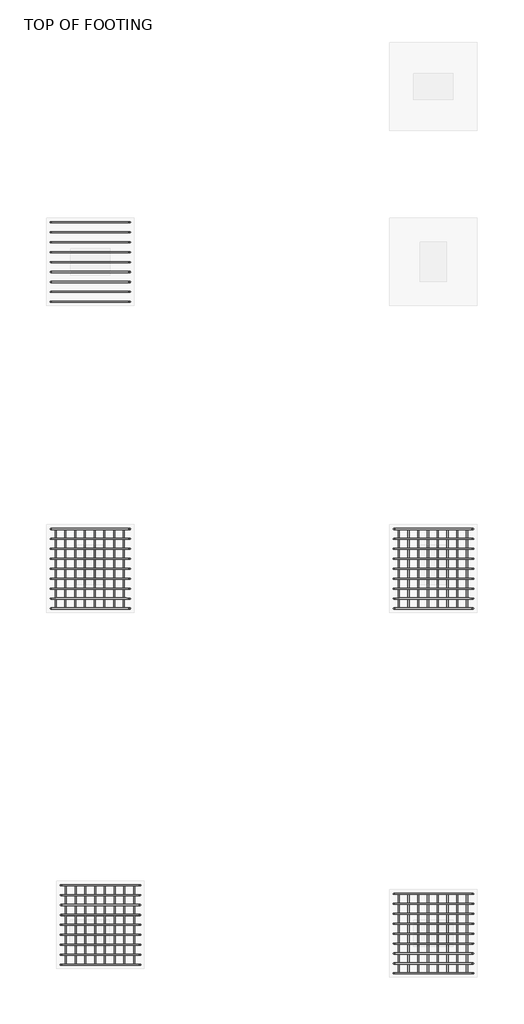
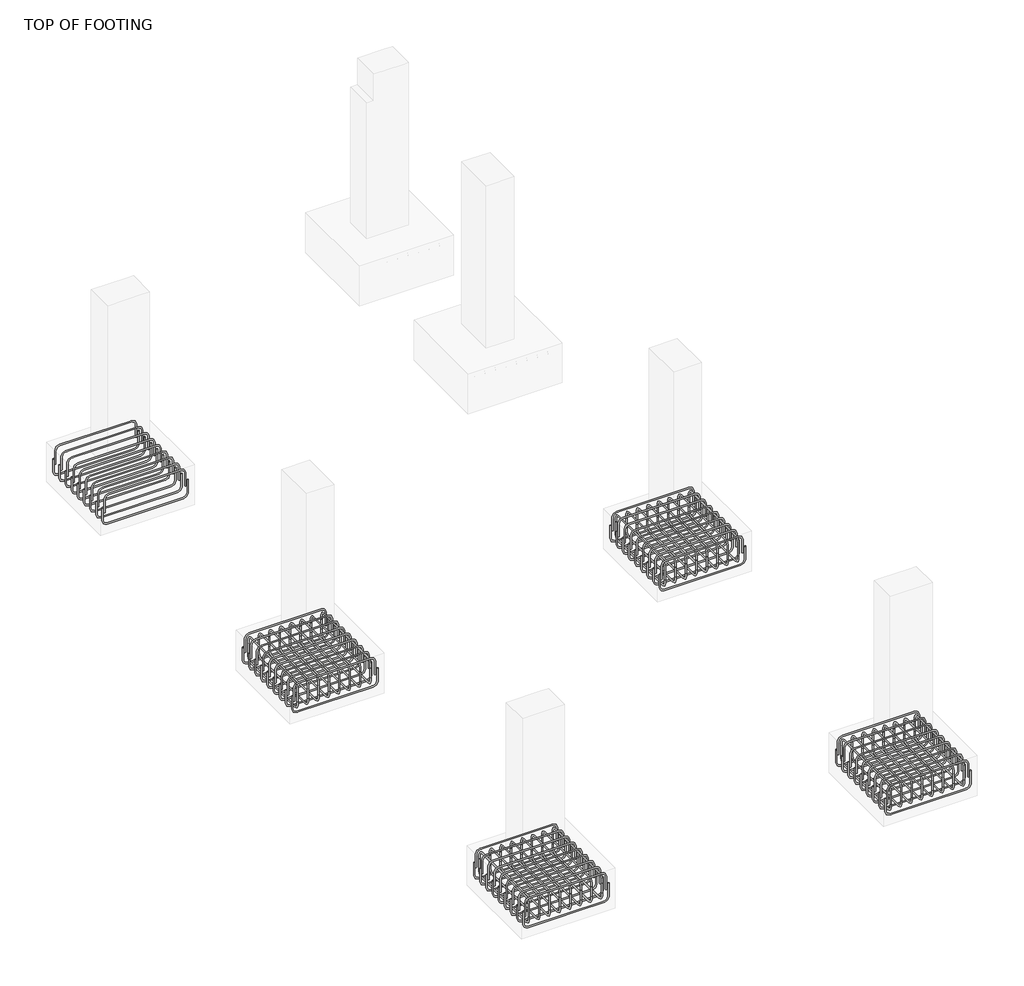
# One storey, part 3 of 20: 18 reinforcing bars.
"""IFC4 building model written with IfcOpenShell, lengths in millimetres."""

from ifc_helpers import new_model, si_unit, point, frame, origin, place, context, project, spatial, polyline, circle_curve, trimmed, segment, composite_curve, source, transform, mapped, element, save
from ifc_brep_helpers import swept_disk

model = new_model("IFC4")

# Units and contexts
model_context = context("Model", 3, world=origin())
ifc_project = project(units=[si_unit("LENGTHUNIT", "METRE", prefix="MILLI")], contexts=[model_context])

# Site, building, storey
site = spatial("IfcSite", under=ifc_project)
building = spatial("IfcBuilding", under=site)
storey = spatial("IfcBuildingStorey", under=building, Name="TOP OF FOOTING", Elevation=-1828.8)

# Reinforcing bars
placement = place(None, origin())
reinforcing_bar_shape = source(origin(), model_context, "Body", "SolidModel", [
    swept_disk(composite_curve([segment(polyline([(-5285.1605653, -11304.2470059, -2006.6587682), (-5285.1605653, -11304.2470059, -2153.9587682)]), True, "CONTINUOUS"), segment(trimmed(circle_curve(frame((-5331.5105653, -11304.2470059, -2153.9587682), z_axis=(0.0, 1.0, 0.0), x_axis=(46.350000000000364, 0.0, 0.0)), 46.35), [point((-5285.1605653, -11304.2470059, -2153.9587682))], [point((-5331.5105653, -11304.2470059, -2200.3087682))], True, "CARTESIAN"), True, "CONTINUOUS"), segment(polyline([(-5331.5105653, -11304.2470059, -2200.3087682), (-6146.1105653, -11304.2470059, -2200.3087682)]), True, "CONTINUOUS"), segment(trimmed(circle_curve(frame((-6146.1105653, -11304.2470059, -2153.9587682), z_axis=(0.0, 1.0, 0.0), x_axis=(0.0, 0.0, -46.34999999999991)), 46.35), [point((-6146.1105653, -11304.2470059, -2200.3087682))], [point((-6192.4605653, -11304.2470059, -2153.9587682))], True, "CARTESIAN"), True, "CONTINUOUS"), segment(polyline([(-6192.4605653, -11304.2470059, -2153.9587682), (-6192.4605653, -11304.2470059, -2006.6587682)]), True, "CONTINUOUS")], self_intersect=False), 6.35),
])
element("IfcReinforcingBar", 1, at=placement, inside=storey, context=model_context, shape_type="MappedRepresentation", body=[
    mapped(reinforcing_bar_shape, transform((0.0, 0.0, 0.0), x_axis=(1.0, 0.0, 0.0), y_axis=(0.0, 1.0, 0.0), z_axis=(0.0, 0.0, 1.0))),
    mapped(reinforcing_bar_shape, transform((0.0, -113.4125, 0.0), x_axis=(1.0, 0.0, 0.0), y_axis=(0.0, 1.0, 0.0), z_axis=(0.0, 0.0, 1.0))),
    mapped(reinforcing_bar_shape, transform((0.0, -226.825, 0.0), x_axis=(1.0, 0.0, 0.0), y_axis=(0.0, 1.0, 0.0), z_axis=(0.0, 0.0, 1.0))),
    mapped(reinforcing_bar_shape, transform((0.0, -340.2375, 0.0), x_axis=(1.0, 0.0, 0.0), y_axis=(0.0, 1.0, 0.0), z_axis=(0.0, 0.0, 1.0))),
    mapped(reinforcing_bar_shape, transform((0.0, -453.65, 0.0), x_axis=(1.0, 0.0, 0.0), y_axis=(0.0, 1.0, 0.0), z_axis=(0.0, 0.0, 1.0))),
    mapped(reinforcing_bar_shape, transform((0.0, -567.0625, 0.0), x_axis=(1.0, 0.0, 0.0), y_axis=(0.0, 1.0, 0.0), z_axis=(0.0, 0.0, 1.0))),
    mapped(reinforcing_bar_shape, transform((0.0, -680.475, 0.0), x_axis=(1.0, 0.0, 0.0), y_axis=(0.0, 1.0, 0.0), z_axis=(0.0, 0.0, 1.0))),
    mapped(reinforcing_bar_shape, transform((0.0, -793.8875, 0.0), x_axis=(1.0, 0.0, 0.0), y_axis=(0.0, 1.0, 0.0), z_axis=(0.0, 0.0, 1.0))),
    mapped(reinforcing_bar_shape, transform((0.0, -907.3, 0.0), x_axis=(1.0, 0.0, 0.0), y_axis=(0.0, 1.0, 0.0), z_axis=(0.0, 0.0, 1.0))),
])
reinforcing_bar_2_shape = source(origin(), model_context, "Body", "SolidModel", [
    swept_disk(composite_curve([segment(polyline([(-6172.986454, -11304.2470059, -2068.8), (-6172.986454, -11304.2470059, -1921.5)]), True, "CONTINUOUS"), segment(trimmed(circle_curve(frame((-6126.636454, -11304.2470059, -1921.5), z_axis=(0.0, 1.0, 0.0), x_axis=(-46.349999999999454, 0.0, 0.0)), 46.35), [point((-6172.986454, -11304.2470059, -1921.5))], [point((-6126.636454, -11304.2470059, -1875.15))], True, "CARTESIAN"), True, "CONTINUOUS"), segment(polyline([(-6126.636454, -11304.2470059, -1875.15), (-5357.1730543, -11304.2470059, -1875.15)]), True, "CONTINUOUS"), segment(trimmed(circle_curve(frame((-5357.1730543, -11304.2470059, -1921.5), z_axis=(0.0, 1.0, 0.0), x_axis=(0.0, 0.0, 46.34999999999991)), 46.35), [point((-5357.1730543, -11304.2470059, -1875.15))], [point((-5310.8230543, -11304.2470059, -1921.5))], True, "CARTESIAN"), True, "CONTINUOUS"), segment(polyline([(-5310.8230543, -11304.2470059, -1921.5), (-5310.8230543, -11304.2470059, -2068.8)]), True, "CONTINUOUS")], self_intersect=False), 6.35),
])
element("IfcReinforcingBar", 2, at=placement, inside=storey, context=model_context, shape_type="MappedRepresentation", body=[
    mapped(reinforcing_bar_2_shape, transform((0.0, 0.0, 0.0), x_axis=(1.0, 0.0, 0.0), y_axis=(0.0, 1.0, 0.0), z_axis=(0.0, 0.0, 1.0))),
    mapped(reinforcing_bar_2_shape, transform((0.0, -113.4125, 0.0), x_axis=(1.0, 0.0, 0.0), y_axis=(0.0, 1.0, 0.0), z_axis=(0.0, 0.0, 1.0))),
    mapped(reinforcing_bar_2_shape, transform((0.0, -226.825, 0.0), x_axis=(1.0, 0.0, 0.0), y_axis=(0.0, 1.0, 0.0), z_axis=(0.0, 0.0, 1.0))),
    mapped(reinforcing_bar_2_shape, transform((0.0, -340.2375, 0.0), x_axis=(1.0, 0.0, 0.0), y_axis=(0.0, 1.0, 0.0), z_axis=(0.0, 0.0, 1.0))),
    mapped(reinforcing_bar_2_shape, transform((0.0, -453.65, 0.0), x_axis=(1.0, 0.0, 0.0), y_axis=(0.0, 1.0, 0.0), z_axis=(0.0, 0.0, 1.0))),
    mapped(reinforcing_bar_2_shape, transform((0.0, -567.0625, 0.0), x_axis=(1.0, 0.0, 0.0), y_axis=(0.0, 1.0, 0.0), z_axis=(0.0, 0.0, 1.0))),
    mapped(reinforcing_bar_2_shape, transform((0.0, -680.475, 0.0), x_axis=(1.0, 0.0, 0.0), y_axis=(0.0, 1.0, 0.0), z_axis=(0.0, 0.0, 1.0))),
    mapped(reinforcing_bar_2_shape, transform((0.0, -793.8875, 0.0), x_axis=(1.0, 0.0, 0.0), y_axis=(0.0, 1.0, 0.0), z_axis=(0.0, 0.0, 1.0))),
    mapped(reinforcing_bar_2_shape, transform((0.0, -907.3, 0.0), x_axis=(1.0, 0.0, 0.0), y_axis=(0.0, 1.0, 0.0), z_axis=(0.0, 0.0, 1.0))),
])
reinforcing_bar_3_shape = source(origin(), model_context, "Body", "SolidModel", [
    swept_disk(composite_curve([segment(polyline([(-5285.1605653, -14804.2470059, -2006.6587682), (-5285.1605653, -14804.2470059, -2153.9587682)]), True, "CONTINUOUS"), segment(trimmed(circle_curve(frame((-5331.5105653, -14804.2470059, -2153.9587682), z_axis=(0.0, 1.0, 0.0), x_axis=(46.350000000000364, 0.0, 0.0)), 46.35), [point((-5285.1605653, -14804.2470059, -2153.9587682))], [point((-5331.5105653, -14804.2470059, -2200.3087682))], True, "CARTESIAN"), True, "CONTINUOUS"), segment(polyline([(-5331.5105653, -14804.2470059, -2200.3087682), (-6146.1105653, -14804.2470059, -2200.3087682)]), True, "CONTINUOUS"), segment(trimmed(circle_curve(frame((-6146.1105653, -14804.2470059, -2153.9587682), z_axis=(0.0, 1.0, 0.0), x_axis=(0.0, 0.0, -46.34999999999991)), 46.35), [point((-6146.1105653, -14804.2470059, -2200.3087682))], [point((-6192.4605653, -14804.2470059, -2153.9587682))], True, "CARTESIAN"), True, "CONTINUOUS"), segment(polyline([(-6192.4605653, -14804.2470059, -2153.9587682), (-6192.4605653, -14804.2470059, -2006.6587682)]), True, "CONTINUOUS")], self_intersect=False), 6.35),
])
element("IfcReinforcingBar", 3, at=placement, inside=storey, context=model_context, shape_type="MappedRepresentation", body=[
    mapped(reinforcing_bar_3_shape, transform((0.0, 0.0, 0.0), x_axis=(1.0, 0.0, 0.0), y_axis=(0.0, 1.0, 0.0), z_axis=(0.0, 0.0, 1.0))),
    mapped(reinforcing_bar_3_shape, transform((0.0, -113.4125, 0.0), x_axis=(1.0, 0.0, 0.0), y_axis=(0.0, 1.0, 0.0), z_axis=(0.0, 0.0, 1.0))),
    mapped(reinforcing_bar_3_shape, transform((0.0, -226.825, 0.0), x_axis=(1.0, 0.0, 0.0), y_axis=(0.0, 1.0, 0.0), z_axis=(0.0, 0.0, 1.0))),
    mapped(reinforcing_bar_3_shape, transform((0.0, -340.2375, 0.0), x_axis=(1.0, 0.0, 0.0), y_axis=(0.0, 1.0, 0.0), z_axis=(0.0, 0.0, 1.0))),
    mapped(reinforcing_bar_3_shape, transform((0.0, -453.65, 0.0), x_axis=(1.0, 0.0, 0.0), y_axis=(0.0, 1.0, 0.0), z_axis=(0.0, 0.0, 1.0))),
    mapped(reinforcing_bar_3_shape, transform((0.0, -567.0625, 0.0), x_axis=(1.0, 0.0, 0.0), y_axis=(0.0, 1.0, 0.0), z_axis=(0.0, 0.0, 1.0))),
    mapped(reinforcing_bar_3_shape, transform((0.0, -680.475, 0.0), x_axis=(1.0, 0.0, 0.0), y_axis=(0.0, 1.0, 0.0), z_axis=(0.0, 0.0, 1.0))),
    mapped(reinforcing_bar_3_shape, transform((0.0, -793.8875, 0.0), x_axis=(1.0, 0.0, 0.0), y_axis=(0.0, 1.0, 0.0), z_axis=(0.0, 0.0, 1.0))),
    mapped(reinforcing_bar_3_shape, transform((0.0, -907.3, 0.0), x_axis=(1.0, 0.0, 0.0), y_axis=(0.0, 1.0, 0.0), z_axis=(0.0, 0.0, 1.0))),
])
reinforcing_bar_4_shape = source(origin(), model_context, "Body", "SolidModel", [
    swept_disk(composite_curve([segment(polyline([(-6172.986454, -14804.2470059, -2068.8), (-6172.986454, -14804.2470059, -1921.5)]), True, "CONTINUOUS"), segment(trimmed(circle_curve(frame((-6126.636454, -14804.2470059, -1921.5), z_axis=(0.0, 1.0, 0.0), x_axis=(-46.349999999999454, 0.0, 0.0)), 46.35), [point((-6172.986454, -14804.2470059, -1921.5))], [point((-6126.636454, -14804.2470059, -1875.15))], True, "CARTESIAN"), True, "CONTINUOUS"), segment(polyline([(-6126.636454, -14804.2470059, -1875.15), (-5357.1730543, -14804.2470059, -1875.15)]), True, "CONTINUOUS"), segment(trimmed(circle_curve(frame((-5357.1730543, -14804.2470059, -1921.5), z_axis=(0.0, 1.0, 0.0), x_axis=(0.0, 0.0, 46.34999999999991)), 46.35), [point((-5357.1730543, -14804.2470059, -1875.15))], [point((-5310.8230543, -14804.2470059, -1921.5))], True, "CARTESIAN"), True, "CONTINUOUS"), segment(polyline([(-5310.8230543, -14804.2470059, -1921.5), (-5310.8230543, -14804.2470059, -2068.8)]), True, "CONTINUOUS")], self_intersect=False), 6.35),
])
element("IfcReinforcingBar", 4, at=placement, inside=storey, context=model_context, shape_type="MappedRepresentation", body=[
    mapped(reinforcing_bar_4_shape, transform((0.0, 0.0, 0.0), x_axis=(1.0, 0.0, 0.0), y_axis=(0.0, 1.0, 0.0), z_axis=(0.0, 0.0, 1.0))),
    mapped(reinforcing_bar_4_shape, transform((0.0, -113.4125, 0.0), x_axis=(1.0, 0.0, 0.0), y_axis=(0.0, 1.0, 0.0), z_axis=(0.0, 0.0, 1.0))),
    mapped(reinforcing_bar_4_shape, transform((0.0, -226.825, 0.0), x_axis=(1.0, 0.0, 0.0), y_axis=(0.0, 1.0, 0.0), z_axis=(0.0, 0.0, 1.0))),
    mapped(reinforcing_bar_4_shape, transform((0.0, -340.2375, 0.0), x_axis=(1.0, 0.0, 0.0), y_axis=(0.0, 1.0, 0.0), z_axis=(0.0, 0.0, 1.0))),
    mapped(reinforcing_bar_4_shape, transform((0.0, -453.65, 0.0), x_axis=(1.0, 0.0, 0.0), y_axis=(0.0, 1.0, 0.0), z_axis=(0.0, 0.0, 1.0))),
    mapped(reinforcing_bar_4_shape, transform((0.0, -567.0625, 0.0), x_axis=(1.0, 0.0, 0.0), y_axis=(0.0, 1.0, 0.0), z_axis=(0.0, 0.0, 1.0))),
    mapped(reinforcing_bar_4_shape, transform((0.0, -680.475, 0.0), x_axis=(1.0, 0.0, 0.0), y_axis=(0.0, 1.0, 0.0), z_axis=(0.0, 0.0, 1.0))),
    mapped(reinforcing_bar_4_shape, transform((0.0, -793.8875, 0.0), x_axis=(1.0, 0.0, 0.0), y_axis=(0.0, 1.0, 0.0), z_axis=(0.0, 0.0, 1.0))),
    mapped(reinforcing_bar_4_shape, transform((0.0, -907.3, 0.0), x_axis=(1.0, 0.0, 0.0), y_axis=(0.0, 1.0, 0.0), z_axis=(0.0, 0.0, 1.0))),
])
reinforcing_bar_5_shape = source(origin(), model_context, "Body", "SolidModel", [
    swept_disk(composite_curve([segment(polyline([(-5356.6575267, -14804.2470059, -2086.1951968), (-5356.6575267, -14804.2470059, -1938.8951968)]), True, "CONTINUOUS"), segment(trimmed(circle_curve(frame((-5356.6575267, -14850.5970059, -1938.8951968), z_axis=(1.0, 0.0, 0.0), x_axis=(0.0, 46.349999999998545, 0.0)), 46.35), [point((-5356.6575267, -14804.2470059, -1938.8951968))], [point((-5356.6575267, -14850.5970059, -1892.5451968))], True, "CARTESIAN"), True, "CONTINUOUS"), segment(polyline([(-5356.6575267, -14850.5970059, -1892.5451968), (-5356.6575267, -15665.1970059, -1892.5451968)]), True, "CONTINUOUS"), segment(trimmed(circle_curve(frame((-5356.6575267, -15665.1970059, -1938.8951968), z_axis=(1.0, 0.0, 0.0), x_axis=(0.0, 0.0, 46.34999999999991)), 46.35), [point((-5356.6575267, -15665.1970059, -1892.5451968))], [point((-5356.6575267, -15711.5470059, -1938.8951968))], True, "CARTESIAN"), True, "CONTINUOUS"), segment(polyline([(-5356.6575267, -15711.5470059, -1938.8951968), (-5356.6575267, -15711.5470059, -2086.1951968)]), True, "CONTINUOUS")], self_intersect=False), 6.35),
])
element("IfcReinforcingBar", 5, at=placement, inside=storey, context=model_context, shape_type="MappedRepresentation", body=[
    mapped(reinforcing_bar_5_shape, transform((0.0, 0.0, 0.0), x_axis=(1.0, 0.0, 0.0), y_axis=(0.0, 1.0, 0.0), z_axis=(0.0, 0.0, 1.0))),
    mapped(reinforcing_bar_5_shape, transform((-111.2862402, 0.0, 0.0), x_axis=(1.0, 0.0, 0.0), y_axis=(0.0, 1.0, 0.0), z_axis=(0.0, 0.0, 1.0))),
    mapped(reinforcing_bar_5_shape, transform((-222.5724804, 0.0, 0.0), x_axis=(1.0, 0.0, 0.0), y_axis=(0.0, 1.0, 0.0), z_axis=(0.0, 0.0, 1.0))),
    mapped(reinforcing_bar_5_shape, transform((-333.8587205, 0.0, 0.0), x_axis=(1.0, 0.0, 0.0), y_axis=(0.0, 1.0, 0.0), z_axis=(0.0, 0.0, 1.0))),
    mapped(reinforcing_bar_5_shape, transform((-445.1449607, 0.0, 0.0), x_axis=(1.0, 0.0, 0.0), y_axis=(0.0, 1.0, 0.0), z_axis=(0.0, 0.0, 1.0))),
    mapped(reinforcing_bar_5_shape, transform((-556.4312009, 0.0, 0.0), x_axis=(1.0, 0.0, 0.0), y_axis=(0.0, 1.0, 0.0), z_axis=(0.0, 0.0, 1.0))),
    mapped(reinforcing_bar_5_shape, transform((-667.7174411, 0.0, 0.0), x_axis=(1.0, 0.0, 0.0), y_axis=(0.0, 1.0, 0.0), z_axis=(0.0, 0.0, 1.0))),
    mapped(reinforcing_bar_5_shape, transform((-779.0036813, 0.0, 0.0), x_axis=(1.0, 0.0, 0.0), y_axis=(0.0, 1.0, 0.0), z_axis=(0.0, 0.0, 1.0))),
])
reinforcing_bar_6_shape = source(origin(), model_context, "Body", "SolidModel", [
    swept_disk(composite_curve([segment(polyline([(-6135.661208, -14804.2470059, -1979.1645013), (-6135.661208, -14804.2470059, -2126.4645013)]), True, "CONTINUOUS"), segment(trimmed(circle_curve(frame((-6135.661208, -14850.5970059, -2126.4645013), z_axis=(-1.0, 0.0, 0.0), x_axis=(0.0, 46.349999999998545, 0.0)), 46.35), [point((-6135.661208, -14804.2470059, -2126.4645013))], [point((-6135.661208, -14850.5970059, -2172.8145013))], True, "CARTESIAN"), True, "CONTINUOUS"), segment(polyline([(-6135.661208, -14850.5970059, -2172.8145013), (-6135.661208, -15665.1970059, -2172.8145013)]), True, "CONTINUOUS"), segment(trimmed(circle_curve(frame((-6135.661208, -15665.1970059, -2126.4645013), z_axis=(-1.0, 0.0, 0.0), x_axis=(0.0, 0.0, -46.34999999999991)), 46.35), [point((-6135.661208, -15665.1970059, -2172.8145013))], [point((-6135.661208, -15711.5470059, -2126.4645013))], True, "CARTESIAN"), True, "CONTINUOUS"), segment(polyline([(-6135.661208, -15711.5470059, -2126.4645013), (-6135.661208, -15711.5470059, -1979.1645013)]), True, "CONTINUOUS")], self_intersect=False), 6.35),
])
element("IfcReinforcingBar", 6, at=placement, inside=storey, context=model_context, shape_type="MappedRepresentation", body=[
    mapped(reinforcing_bar_6_shape, transform((0.0, 0.0, 0.0), x_axis=(1.0, 0.0, 0.0), y_axis=(0.0, 1.0, 0.0), z_axis=(0.0, 0.0, 1.0))),
    mapped(reinforcing_bar_6_shape, transform((111.2862402, 0.0, 0.0), x_axis=(1.0, 0.0, 0.0), y_axis=(0.0, 1.0, 0.0), z_axis=(0.0, 0.0, 1.0))),
    mapped(reinforcing_bar_6_shape, transform((222.5724804, 0.0, 0.0), x_axis=(1.0, 0.0, 0.0), y_axis=(0.0, 1.0, 0.0), z_axis=(0.0, 0.0, 1.0))),
    mapped(reinforcing_bar_6_shape, transform((333.8587205, 0.0, 0.0), x_axis=(1.0, 0.0, 0.0), y_axis=(0.0, 1.0, 0.0), z_axis=(0.0, 0.0, 1.0))),
    mapped(reinforcing_bar_6_shape, transform((445.1449607, 0.0, 0.0), x_axis=(1.0, 0.0, 0.0), y_axis=(0.0, 1.0, 0.0), z_axis=(0.0, 0.0, 1.0))),
    mapped(reinforcing_bar_6_shape, transform((556.4312009, 0.0, 0.0), x_axis=(1.0, 0.0, 0.0), y_axis=(0.0, 1.0, 0.0), z_axis=(0.0, 0.0, 1.0))),
    mapped(reinforcing_bar_6_shape, transform((667.7174411, 0.0, 0.0), x_axis=(1.0, 0.0, 0.0), y_axis=(0.0, 1.0, 0.0), z_axis=(0.0, 0.0, 1.0))),
    mapped(reinforcing_bar_6_shape, transform((779.0036813, 0.0, 0.0), x_axis=(1.0, 0.0, 0.0), y_axis=(0.0, 1.0, 0.0), z_axis=(0.0, 0.0, 1.0))),
])
reinforcing_bar_7_shape = source(origin(), model_context, "Body", "SolidModel", [
    swept_disk(composite_curve([segment(polyline([(-5168.1365686, -18868.8804373, -2006.6587682), (-5168.1365686, -18868.8804373, -2153.9587682)]), True, "CONTINUOUS"), segment(trimmed(circle_curve(frame((-5214.4865686, -18868.8804373, -2153.9587682), z_axis=(0.0, 1.0, 0.0), x_axis=(46.350000000000364, 0.0, 0.0)), 46.35), [point((-5168.1365686, -18868.8804373, -2153.9587682))], [point((-5214.4865686, -18868.8804373, -2200.3087682))], True, "CARTESIAN"), True, "CONTINUOUS"), segment(polyline([(-5214.4865686, -18868.8804373, -2200.3087682), (-6029.0865686, -18868.8804373, -2200.3087682)]), True, "CONTINUOUS"), segment(trimmed(circle_curve(frame((-6029.0865686, -18868.8804373, -2153.9587682), z_axis=(0.0, 1.0, 0.0), x_axis=(0.0, 0.0, -46.34999999999991)), 46.35), [point((-6029.0865686, -18868.8804373, -2200.3087682))], [point((-6075.4365686, -18868.8804373, -2153.9587682))], True, "CARTESIAN"), True, "CONTINUOUS"), segment(polyline([(-6075.4365686, -18868.8804373, -2153.9587682), (-6075.4365686, -18868.8804373, -2006.6587682)]), True, "CONTINUOUS")], self_intersect=False), 6.35),
])
element("IfcReinforcingBar", 7, at=placement, inside=storey, context=model_context, shape_type="MappedRepresentation", body=[
    mapped(reinforcing_bar_7_shape, transform((0.0, 0.0, 0.0), x_axis=(1.0, 0.0, 0.0), y_axis=(0.0, 1.0, 0.0), z_axis=(0.0, 0.0, 1.0))),
    mapped(reinforcing_bar_7_shape, transform((0.0, -113.4125, 0.0), x_axis=(1.0, 0.0, 0.0), y_axis=(0.0, 1.0, 0.0), z_axis=(0.0, 0.0, 1.0))),
    mapped(reinforcing_bar_7_shape, transform((0.0, -226.825, 0.0), x_axis=(1.0, 0.0, 0.0), y_axis=(0.0, 1.0, 0.0), z_axis=(0.0, 0.0, 1.0))),
    mapped(reinforcing_bar_7_shape, transform((0.0, -340.2375, 0.0), x_axis=(1.0, 0.0, 0.0), y_axis=(0.0, 1.0, 0.0), z_axis=(0.0, 0.0, 1.0))),
    mapped(reinforcing_bar_7_shape, transform((0.0, -453.65, 0.0), x_axis=(1.0, 0.0, 0.0), y_axis=(0.0, 1.0, 0.0), z_axis=(0.0, 0.0, 1.0))),
    mapped(reinforcing_bar_7_shape, transform((0.0, -567.0625, 0.0), x_axis=(1.0, 0.0, 0.0), y_axis=(0.0, 1.0, 0.0), z_axis=(0.0, 0.0, 1.0))),
    mapped(reinforcing_bar_7_shape, transform((0.0, -680.475, 0.0), x_axis=(1.0, 0.0, 0.0), y_axis=(0.0, 1.0, 0.0), z_axis=(0.0, 0.0, 1.0))),
    mapped(reinforcing_bar_7_shape, transform((0.0, -793.8875, 0.0), x_axis=(1.0, 0.0, 0.0), y_axis=(0.0, 1.0, 0.0), z_axis=(0.0, 0.0, 1.0))),
    mapped(reinforcing_bar_7_shape, transform((0.0, -907.3, 0.0), x_axis=(1.0, 0.0, 0.0), y_axis=(0.0, 1.0, 0.0), z_axis=(0.0, 0.0, 1.0))),
])
reinforcing_bar_8_shape = source(origin(), model_context, "Body", "SolidModel", [
    swept_disk(composite_curve([segment(polyline([(-6055.9624573, -18868.8804373, -2068.8), (-6055.9624573, -18868.8804373, -1921.5)]), True, "CONTINUOUS"), segment(trimmed(circle_curve(frame((-6009.6124573, -18868.8804373, -1921.5), z_axis=(0.0, 1.0, 0.0), x_axis=(-46.350000000000364, 0.0, 0.0)), 46.35), [point((-6055.9624573, -18868.8804373, -1921.5))], [point((-6009.6124573, -18868.8804373, -1875.15))], True, "CARTESIAN"), True, "CONTINUOUS"), segment(polyline([(-6009.6124573, -18868.8804373, -1875.15), (-5240.1490576, -18868.8804373, -1875.15)]), True, "CONTINUOUS"), segment(trimmed(circle_curve(frame((-5240.1490576, -18868.8804373, -1921.5), z_axis=(0.0, 1.0, 0.0), x_axis=(0.0, 0.0, 46.34999999999991)), 46.35), [point((-5240.1490576, -18868.8804373, -1875.15))], [point((-5193.7990576, -18868.8804373, -1921.5))], True, "CARTESIAN"), True, "CONTINUOUS"), segment(polyline([(-5193.7990576, -18868.8804373, -1921.5), (-5193.7990576, -18868.8804373, -2068.8)]), True, "CONTINUOUS")], self_intersect=False), 6.35),
])
element("IfcReinforcingBar", 8, at=placement, inside=storey, context=model_context, shape_type="MappedRepresentation", body=[
    mapped(reinforcing_bar_8_shape, transform((0.0, 0.0, 0.0), x_axis=(1.0, 0.0, 0.0), y_axis=(0.0, 1.0, 0.0), z_axis=(0.0, 0.0, 1.0))),
    mapped(reinforcing_bar_8_shape, transform((0.0, -113.4125, 0.0), x_axis=(1.0, 0.0, 0.0), y_axis=(0.0, 1.0, 0.0), z_axis=(0.0, 0.0, 1.0))),
    mapped(reinforcing_bar_8_shape, transform((0.0, -226.825, 0.0), x_axis=(1.0, 0.0, 0.0), y_axis=(0.0, 1.0, 0.0), z_axis=(0.0, 0.0, 1.0))),
    mapped(reinforcing_bar_8_shape, transform((0.0, -340.2375, 0.0), x_axis=(1.0, 0.0, 0.0), y_axis=(0.0, 1.0, 0.0), z_axis=(0.0, 0.0, 1.0))),
    mapped(reinforcing_bar_8_shape, transform((0.0, -453.65, 0.0), x_axis=(1.0, 0.0, 0.0), y_axis=(0.0, 1.0, 0.0), z_axis=(0.0, 0.0, 1.0))),
    mapped(reinforcing_bar_8_shape, transform((0.0, -567.0625, 0.0), x_axis=(1.0, 0.0, 0.0), y_axis=(0.0, 1.0, 0.0), z_axis=(0.0, 0.0, 1.0))),
    mapped(reinforcing_bar_8_shape, transform((0.0, -680.475, 0.0), x_axis=(1.0, 0.0, 0.0), y_axis=(0.0, 1.0, 0.0), z_axis=(0.0, 0.0, 1.0))),
    mapped(reinforcing_bar_8_shape, transform((0.0, -793.8875, 0.0), x_axis=(1.0, 0.0, 0.0), y_axis=(0.0, 1.0, 0.0), z_axis=(0.0, 0.0, 1.0))),
    mapped(reinforcing_bar_8_shape, transform((0.0, -907.3, 0.0), x_axis=(1.0, 0.0, 0.0), y_axis=(0.0, 1.0, 0.0), z_axis=(0.0, 0.0, 1.0))),
])
reinforcing_bar_9_shape = source(origin(), model_context, "Body", "SolidModel", [
    swept_disk(composite_curve([segment(polyline([(-5239.63353, -18868.8804373, -2086.1951968), (-5239.63353, -18868.8804373, -1938.8951968)]), True, "CONTINUOUS"), segment(trimmed(circle_curve(frame((-5239.63353, -18915.2304373, -1938.8951968), z_axis=(1.0, 0.0, 0.0), x_axis=(0.0, 46.35000000000218, 0.0)), 46.35), [point((-5239.63353, -18868.8804373, -1938.8951968))], [point((-5239.63353, -18915.2304373, -1892.5451968))], True, "CARTESIAN"), True, "CONTINUOUS"), segment(polyline([(-5239.63353, -18915.2304373, -1892.5451968), (-5239.63353, -19729.8304373, -1892.5451968)]), True, "CONTINUOUS"), segment(trimmed(circle_curve(frame((-5239.63353, -19729.8304373, -1938.8951968), z_axis=(1.0, 0.0, 0.0), x_axis=(0.0, 0.0, 46.34999999999991)), 46.35), [point((-5239.63353, -19729.8304373, -1892.5451968))], [point((-5239.63353, -19776.1804373, -1938.8951968))], True, "CARTESIAN"), True, "CONTINUOUS"), segment(polyline([(-5239.63353, -19776.1804373, -1938.8951968), (-5239.63353, -19776.1804373, -2086.1951968)]), True, "CONTINUOUS")], self_intersect=False), 6.35),
])
element("IfcReinforcingBar", 9, at=placement, inside=storey, context=model_context, shape_type="MappedRepresentation", body=[
    mapped(reinforcing_bar_9_shape, transform((0.0, 0.0, 0.0), x_axis=(1.0, 0.0, 0.0), y_axis=(0.0, 1.0, 0.0), z_axis=(0.0, 0.0, 1.0))),
    mapped(reinforcing_bar_9_shape, transform((-111.2862402, 0.0, 0.0), x_axis=(1.0, 0.0, 0.0), y_axis=(0.0, 1.0, 0.0), z_axis=(0.0, 0.0, 1.0))),
    mapped(reinforcing_bar_9_shape, transform((-222.5724804, 0.0, 0.0), x_axis=(1.0, 0.0, 0.0), y_axis=(0.0, 1.0, 0.0), z_axis=(0.0, 0.0, 1.0))),
    mapped(reinforcing_bar_9_shape, transform((-333.8587205, 0.0, 0.0), x_axis=(1.0, 0.0, 0.0), y_axis=(0.0, 1.0, 0.0), z_axis=(0.0, 0.0, 1.0))),
    mapped(reinforcing_bar_9_shape, transform((-445.1449607, 0.0, 0.0), x_axis=(1.0, 0.0, 0.0), y_axis=(0.0, 1.0, 0.0), z_axis=(0.0, 0.0, 1.0))),
    mapped(reinforcing_bar_9_shape, transform((-556.4312009, 0.0, 0.0), x_axis=(1.0, 0.0, 0.0), y_axis=(0.0, 1.0, 0.0), z_axis=(0.0, 0.0, 1.0))),
    mapped(reinforcing_bar_9_shape, transform((-667.7174411, 0.0, 0.0), x_axis=(1.0, 0.0, 0.0), y_axis=(0.0, 1.0, 0.0), z_axis=(0.0, 0.0, 1.0))),
    mapped(reinforcing_bar_9_shape, transform((-779.0036813, 0.0, 0.0), x_axis=(1.0, 0.0, 0.0), y_axis=(0.0, 1.0, 0.0), z_axis=(0.0, 0.0, 1.0))),
])
reinforcing_bar_10_shape = source(origin(), model_context, "Body", "SolidModel", [
    swept_disk(composite_curve([segment(polyline([(-6018.6372113, -18868.8804373, -1979.1645013), (-6018.6372113, -18868.8804373, -2126.4645013)]), True, "CONTINUOUS"), segment(trimmed(circle_curve(frame((-6018.6372113, -18915.2304373, -2126.4645013), z_axis=(-1.0, 0.0, 0.0), x_axis=(0.0, 46.35000000000218, 0.0)), 46.35), [point((-6018.6372113, -18868.8804373, -2126.4645013))], [point((-6018.6372113, -18915.2304373, -2172.8145013))], True, "CARTESIAN"), True, "CONTINUOUS"), segment(polyline([(-6018.6372113, -18915.2304373, -2172.8145013), (-6018.6372113, -19729.8304373, -2172.8145013)]), True, "CONTINUOUS"), segment(trimmed(circle_curve(frame((-6018.6372113, -19729.8304373, -2126.4645013), z_axis=(-1.0, 0.0, 0.0), x_axis=(0.0, 0.0, -46.34999999999991)), 46.35), [point((-6018.6372113, -19729.8304373, -2172.8145013))], [point((-6018.6372113, -19776.1804373, -2126.4645013))], True, "CARTESIAN"), True, "CONTINUOUS"), segment(polyline([(-6018.6372113, -19776.1804373, -2126.4645013), (-6018.6372113, -19776.1804373, -1979.1645013)]), True, "CONTINUOUS")], self_intersect=False), 6.35),
])
element("IfcReinforcingBar", 10, at=placement, inside=storey, context=model_context, shape_type="MappedRepresentation", body=[
    mapped(reinforcing_bar_10_shape, transform((0.0, 0.0, 0.0), x_axis=(1.0, 0.0, 0.0), y_axis=(0.0, 1.0, 0.0), z_axis=(0.0, 0.0, 1.0))),
    mapped(reinforcing_bar_10_shape, transform((111.2862402, 0.0, 0.0), x_axis=(1.0, 0.0, 0.0), y_axis=(0.0, 1.0, 0.0), z_axis=(0.0, 0.0, 1.0))),
    mapped(reinforcing_bar_10_shape, transform((222.5724804, 0.0, 0.0), x_axis=(1.0, 0.0, 0.0), y_axis=(0.0, 1.0, 0.0), z_axis=(0.0, 0.0, 1.0))),
    mapped(reinforcing_bar_10_shape, transform((333.8587205, 0.0, 0.0), x_axis=(1.0, 0.0, 0.0), y_axis=(0.0, 1.0, 0.0), z_axis=(0.0, 0.0, 1.0))),
    mapped(reinforcing_bar_10_shape, transform((445.1449607, 0.0, 0.0), x_axis=(1.0, 0.0, 0.0), y_axis=(0.0, 1.0, 0.0), z_axis=(0.0, 0.0, 1.0))),
    mapped(reinforcing_bar_10_shape, transform((556.4312009, 0.0, 0.0), x_axis=(1.0, 0.0, 0.0), y_axis=(0.0, 1.0, 0.0), z_axis=(0.0, 0.0, 1.0))),
    mapped(reinforcing_bar_10_shape, transform((667.7174411, 0.0, 0.0), x_axis=(1.0, 0.0, 0.0), y_axis=(0.0, 1.0, 0.0), z_axis=(0.0, 0.0, 1.0))),
    mapped(reinforcing_bar_10_shape, transform((779.0036813, 0.0, 0.0), x_axis=(1.0, 0.0, 0.0), y_axis=(0.0, 1.0, 0.0), z_axis=(0.0, 0.0, 1.0))),
])
reinforcing_bar_11_shape = source(origin(), model_context, "Body", "SolidModel", [
    swept_disk(composite_curve([segment(polyline([(-1368.1365686, -18968.8804373, -2006.6587682), (-1368.1365686, -18968.8804373, -2153.9587682)]), True, "CONTINUOUS"), segment(trimmed(circle_curve(frame((-1414.4865686, -18968.8804373, -2153.9587682), z_axis=(0.0, 1.0, 0.0), x_axis=(46.350000000000136, 0.0, 0.0)), 46.35), [point((-1368.1365686, -18968.8804373, -2153.9587682))], [point((-1414.4865686, -18968.8804373, -2200.3087682))], True, "CARTESIAN"), True, "CONTINUOUS"), segment(polyline([(-1414.4865686, -18968.8804373, -2200.3087682), (-2229.0865686, -18968.8804373, -2200.3087682)]), True, "CONTINUOUS"), segment(trimmed(circle_curve(frame((-2229.0865686, -18968.8804373, -2153.9587682), z_axis=(0.0, 1.0, 0.0), x_axis=(0.0, 0.0, -46.34999999999991)), 46.35), [point((-2229.0865686, -18968.8804373, -2200.3087682))], [point((-2275.4365686, -18968.8804373, -2153.9587682))], True, "CARTESIAN"), True, "CONTINUOUS"), segment(polyline([(-2275.4365686, -18968.8804373, -2153.9587682), (-2275.4365686, -18968.8804373, -2006.6587682)]), True, "CONTINUOUS")], self_intersect=False), 6.35),
])
element("IfcReinforcingBar", 11, at=placement, inside=storey, context=model_context, shape_type="MappedRepresentation", body=[
    mapped(reinforcing_bar_11_shape, transform((0.0, 0.0, 0.0), x_axis=(1.0, 0.0, 0.0), y_axis=(0.0, 1.0, 0.0), z_axis=(0.0, 0.0, 1.0))),
    mapped(reinforcing_bar_11_shape, transform((0.0, -113.4125, 0.0), x_axis=(1.0, 0.0, 0.0), y_axis=(0.0, 1.0, 0.0), z_axis=(0.0, 0.0, 1.0))),
    mapped(reinforcing_bar_11_shape, transform((0.0, -226.825, 0.0), x_axis=(1.0, 0.0, 0.0), y_axis=(0.0, 1.0, 0.0), z_axis=(0.0, 0.0, 1.0))),
    mapped(reinforcing_bar_11_shape, transform((0.0, -340.2375, 0.0), x_axis=(1.0, 0.0, 0.0), y_axis=(0.0, 1.0, 0.0), z_axis=(0.0, 0.0, 1.0))),
    mapped(reinforcing_bar_11_shape, transform((0.0, -453.65, 0.0), x_axis=(1.0, 0.0, 0.0), y_axis=(0.0, 1.0, 0.0), z_axis=(0.0, 0.0, 1.0))),
    mapped(reinforcing_bar_11_shape, transform((0.0, -567.0625, 0.0), x_axis=(1.0, 0.0, 0.0), y_axis=(0.0, 1.0, 0.0), z_axis=(0.0, 0.0, 1.0))),
    mapped(reinforcing_bar_11_shape, transform((0.0, -680.475, 0.0), x_axis=(1.0, 0.0, 0.0), y_axis=(0.0, 1.0, 0.0), z_axis=(0.0, 0.0, 1.0))),
    mapped(reinforcing_bar_11_shape, transform((0.0, -793.8875, 0.0), x_axis=(1.0, 0.0, 0.0), y_axis=(0.0, 1.0, 0.0), z_axis=(0.0, 0.0, 1.0))),
    mapped(reinforcing_bar_11_shape, transform((0.0, -907.3, 0.0), x_axis=(1.0, 0.0, 0.0), y_axis=(0.0, 1.0, 0.0), z_axis=(0.0, 0.0, 1.0))),
])
reinforcing_bar_12_shape = source(origin(), model_context, "Body", "SolidModel", [
    swept_disk(composite_curve([segment(polyline([(-2255.9624573, -18968.8804373, -2068.8), (-2255.9624573, -18968.8804373, -1921.5)]), True, "CONTINUOUS"), segment(trimmed(circle_curve(frame((-2209.6124573, -18968.8804373, -1921.5), z_axis=(0.0, 1.0, 0.0), x_axis=(-46.34999999999991, 0.0, 0.0)), 46.35), [point((-2255.9624573, -18968.8804373, -1921.5))], [point((-2209.6124573, -18968.8804373, -1875.15))], True, "CARTESIAN"), True, "CONTINUOUS"), segment(polyline([(-2209.6124573, -18968.8804373, -1875.15), (-1440.1490576, -18968.8804373, -1875.15)]), True, "CONTINUOUS"), segment(trimmed(circle_curve(frame((-1440.1490576, -18968.8804373, -1921.5), z_axis=(0.0, 1.0, 0.0), x_axis=(0.0, 0.0, 46.34999999999991)), 46.35), [point((-1440.1490576, -18968.8804373, -1875.15))], [point((-1393.7990576, -18968.8804373, -1921.5))], True, "CARTESIAN"), True, "CONTINUOUS"), segment(polyline([(-1393.7990576, -18968.8804373, -1921.5), (-1393.7990576, -18968.8804373, -2068.8)]), True, "CONTINUOUS")], self_intersect=False), 6.35),
])
element("IfcReinforcingBar", 12, at=placement, inside=storey, context=model_context, shape_type="MappedRepresentation", body=[
    mapped(reinforcing_bar_12_shape, transform((0.0, 0.0, 0.0), x_axis=(1.0, 0.0, 0.0), y_axis=(0.0, 1.0, 0.0), z_axis=(0.0, 0.0, 1.0))),
    mapped(reinforcing_bar_12_shape, transform((0.0, -113.4125, 0.0), x_axis=(1.0, 0.0, 0.0), y_axis=(0.0, 1.0, 0.0), z_axis=(0.0, 0.0, 1.0))),
    mapped(reinforcing_bar_12_shape, transform((0.0, -226.825, 0.0), x_axis=(1.0, 0.0, 0.0), y_axis=(0.0, 1.0, 0.0), z_axis=(0.0, 0.0, 1.0))),
    mapped(reinforcing_bar_12_shape, transform((0.0, -340.2375, 0.0), x_axis=(1.0, 0.0, 0.0), y_axis=(0.0, 1.0, 0.0), z_axis=(0.0, 0.0, 1.0))),
    mapped(reinforcing_bar_12_shape, transform((0.0, -453.65, 0.0), x_axis=(1.0, 0.0, 0.0), y_axis=(0.0, 1.0, 0.0), z_axis=(0.0, 0.0, 1.0))),
    mapped(reinforcing_bar_12_shape, transform((0.0, -567.0625, 0.0), x_axis=(1.0, 0.0, 0.0), y_axis=(0.0, 1.0, 0.0), z_axis=(0.0, 0.0, 1.0))),
    mapped(reinforcing_bar_12_shape, transform((0.0, -680.475, 0.0), x_axis=(1.0, 0.0, 0.0), y_axis=(0.0, 1.0, 0.0), z_axis=(0.0, 0.0, 1.0))),
    mapped(reinforcing_bar_12_shape, transform((0.0, -793.8875, 0.0), x_axis=(1.0, 0.0, 0.0), y_axis=(0.0, 1.0, 0.0), z_axis=(0.0, 0.0, 1.0))),
    mapped(reinforcing_bar_12_shape, transform((0.0, -907.3, 0.0), x_axis=(1.0, 0.0, 0.0), y_axis=(0.0, 1.0, 0.0), z_axis=(0.0, 0.0, 1.0))),
])
reinforcing_bar_13_shape = source(origin(), model_context, "Body", "SolidModel", [
    swept_disk(composite_curve([segment(polyline([(-1439.63353, -18968.8804373, -2086.1951968), (-1439.63353, -18968.8804373, -1938.8951968)]), True, "CONTINUOUS"), segment(trimmed(circle_curve(frame((-1439.63353, -19015.2304373, -1938.8951968), z_axis=(1.0, 0.0, 0.0), x_axis=(0.0, 46.35000000000218, 0.0)), 46.35), [point((-1439.63353, -18968.8804373, -1938.8951968))], [point((-1439.63353, -19015.2304373, -1892.5451968))], True, "CARTESIAN"), True, "CONTINUOUS"), segment(polyline([(-1439.63353, -19015.2304373, -1892.5451968), (-1439.63353, -19829.8304373, -1892.5451968)]), True, "CONTINUOUS"), segment(trimmed(circle_curve(frame((-1439.63353, -19829.8304373, -1938.8951968), z_axis=(1.0, 0.0, 0.0), x_axis=(0.0, 0.0, 46.34999999999991)), 46.35), [point((-1439.63353, -19829.8304373, -1892.5451968))], [point((-1439.63353, -19876.1804373, -1938.8951968))], True, "CARTESIAN"), True, "CONTINUOUS"), segment(polyline([(-1439.63353, -19876.1804373, -1938.8951968), (-1439.63353, -19876.1804373, -2086.1951968)]), True, "CONTINUOUS")], self_intersect=False), 6.35),
])
element("IfcReinforcingBar", 13, at=placement, inside=storey, context=model_context, shape_type="MappedRepresentation", body=[
    mapped(reinforcing_bar_13_shape, transform((0.0, 0.0, 0.0), x_axis=(1.0, 0.0, 0.0), y_axis=(0.0, 1.0, 0.0), z_axis=(0.0, 0.0, 1.0))),
    mapped(reinforcing_bar_13_shape, transform((-111.2862402, 0.0, 0.0), x_axis=(1.0, 0.0, 0.0), y_axis=(0.0, 1.0, 0.0), z_axis=(0.0, 0.0, 1.0))),
    mapped(reinforcing_bar_13_shape, transform((-222.5724804, 0.0, 0.0), x_axis=(1.0, 0.0, 0.0), y_axis=(0.0, 1.0, 0.0), z_axis=(0.0, 0.0, 1.0))),
    mapped(reinforcing_bar_13_shape, transform((-333.8587205, 0.0, 0.0), x_axis=(1.0, 0.0, 0.0), y_axis=(0.0, 1.0, 0.0), z_axis=(0.0, 0.0, 1.0))),
    mapped(reinforcing_bar_13_shape, transform((-445.1449607, 0.0, 0.0), x_axis=(1.0, 0.0, 0.0), y_axis=(0.0, 1.0, 0.0), z_axis=(0.0, 0.0, 1.0))),
    mapped(reinforcing_bar_13_shape, transform((-556.4312009, 0.0, 0.0), x_axis=(1.0, 0.0, 0.0), y_axis=(0.0, 1.0, 0.0), z_axis=(0.0, 0.0, 1.0))),
    mapped(reinforcing_bar_13_shape, transform((-667.7174411, 0.0, 0.0), x_axis=(1.0, 0.0, 0.0), y_axis=(0.0, 1.0, 0.0), z_axis=(0.0, 0.0, 1.0))),
    mapped(reinforcing_bar_13_shape, transform((-779.0036813, 0.0, 0.0), x_axis=(1.0, 0.0, 0.0), y_axis=(0.0, 1.0, 0.0), z_axis=(0.0, 0.0, 1.0))),
])
reinforcing_bar_14_shape = source(origin(), model_context, "Body", "SolidModel", [
    swept_disk(composite_curve([segment(polyline([(-2218.6372113, -18968.8804373, -1979.1645013), (-2218.6372113, -18968.8804373, -2126.4645013)]), True, "CONTINUOUS"), segment(trimmed(circle_curve(frame((-2218.6372113, -19015.2304373, -2126.4645013), z_axis=(-1.0, 0.0, 0.0), x_axis=(0.0, 46.35000000000218, 0.0)), 46.35), [point((-2218.6372113, -18968.8804373, -2126.4645013))], [point((-2218.6372113, -19015.2304373, -2172.8145013))], True, "CARTESIAN"), True, "CONTINUOUS"), segment(polyline([(-2218.6372113, -19015.2304373, -2172.8145013), (-2218.6372113, -19829.8304373, -2172.8145013)]), True, "CONTINUOUS"), segment(trimmed(circle_curve(frame((-2218.6372113, -19829.8304373, -2126.4645013), z_axis=(-1.0, 0.0, 0.0), x_axis=(0.0, 0.0, -46.34999999999991)), 46.35), [point((-2218.6372113, -19829.8304373, -2172.8145013))], [point((-2218.6372113, -19876.1804373, -2126.4645013))], True, "CARTESIAN"), True, "CONTINUOUS"), segment(polyline([(-2218.6372113, -19876.1804373, -2126.4645013), (-2218.6372113, -19876.1804373, -1979.1645013)]), True, "CONTINUOUS")], self_intersect=False), 6.35),
])
element("IfcReinforcingBar", 14, at=placement, inside=storey, context=model_context, shape_type="MappedRepresentation", body=[
    mapped(reinforcing_bar_14_shape, transform((0.0, 0.0, 0.0), x_axis=(1.0, 0.0, 0.0), y_axis=(0.0, 1.0, 0.0), z_axis=(0.0, 0.0, 1.0))),
    mapped(reinforcing_bar_14_shape, transform((111.2862402, 0.0, 0.0), x_axis=(1.0, 0.0, 0.0), y_axis=(0.0, 1.0, 0.0), z_axis=(0.0, 0.0, 1.0))),
    mapped(reinforcing_bar_14_shape, transform((222.5724804, 0.0, 0.0), x_axis=(1.0, 0.0, 0.0), y_axis=(0.0, 1.0, 0.0), z_axis=(0.0, 0.0, 1.0))),
    mapped(reinforcing_bar_14_shape, transform((333.8587205, 0.0, 0.0), x_axis=(1.0, 0.0, 0.0), y_axis=(0.0, 1.0, 0.0), z_axis=(0.0, 0.0, 1.0))),
    mapped(reinforcing_bar_14_shape, transform((445.1449607, 0.0, 0.0), x_axis=(1.0, 0.0, 0.0), y_axis=(0.0, 1.0, 0.0), z_axis=(0.0, 0.0, 1.0))),
    mapped(reinforcing_bar_14_shape, transform((556.4312009, 0.0, 0.0), x_axis=(1.0, 0.0, 0.0), y_axis=(0.0, 1.0, 0.0), z_axis=(0.0, 0.0, 1.0))),
    mapped(reinforcing_bar_14_shape, transform((667.7174411, 0.0, 0.0), x_axis=(1.0, 0.0, 0.0), y_axis=(0.0, 1.0, 0.0), z_axis=(0.0, 0.0, 1.0))),
    mapped(reinforcing_bar_14_shape, transform((779.0036813, 0.0, 0.0), x_axis=(1.0, 0.0, 0.0), y_axis=(0.0, 1.0, 0.0), z_axis=(0.0, 0.0, 1.0))),
])
reinforcing_bar_15_shape = source(origin(), model_context, "Body", "SolidModel", [
    swept_disk(composite_curve([segment(polyline([(-1368.1365686, -14804.2470059, -2006.6587682), (-1368.1365686, -14804.2470059, -2153.9587682)]), True, "CONTINUOUS"), segment(trimmed(circle_curve(frame((-1414.4865686, -14804.2470059, -2153.9587682), z_axis=(0.0, 1.0, 0.0), x_axis=(46.350000000000136, 0.0, 0.0)), 46.35), [point((-1368.1365686, -14804.2470059, -2153.9587682))], [point((-1414.4865686, -14804.2470059, -2200.3087682))], True, "CARTESIAN"), True, "CONTINUOUS"), segment(polyline([(-1414.4865686, -14804.2470059, -2200.3087682), (-2229.0865686, -14804.2470059, -2200.3087682)]), True, "CONTINUOUS"), segment(trimmed(circle_curve(frame((-2229.0865686, -14804.2470059, -2153.9587682), z_axis=(0.0, 1.0, 0.0), x_axis=(0.0, 0.0, -46.34999999999991)), 46.35), [point((-2229.0865686, -14804.2470059, -2200.3087682))], [point((-2275.4365686, -14804.2470059, -2153.9587682))], True, "CARTESIAN"), True, "CONTINUOUS"), segment(polyline([(-2275.4365686, -14804.2470059, -2153.9587682), (-2275.4365686, -14804.2470059, -2006.6587682)]), True, "CONTINUOUS")], self_intersect=False), 6.35),
])
element("IfcReinforcingBar", 15, at=placement, inside=storey, context=model_context, shape_type="MappedRepresentation", body=[
    mapped(reinforcing_bar_15_shape, transform((0.0, 0.0, 0.0), x_axis=(1.0, 0.0, 0.0), y_axis=(0.0, 1.0, 0.0), z_axis=(0.0, 0.0, 1.0))),
    mapped(reinforcing_bar_15_shape, transform((0.0, -113.4125, 0.0), x_axis=(1.0, 0.0, 0.0), y_axis=(0.0, 1.0, 0.0), z_axis=(0.0, 0.0, 1.0))),
    mapped(reinforcing_bar_15_shape, transform((0.0, -226.825, 0.0), x_axis=(1.0, 0.0, 0.0), y_axis=(0.0, 1.0, 0.0), z_axis=(0.0, 0.0, 1.0))),
    mapped(reinforcing_bar_15_shape, transform((0.0, -340.2375, 0.0), x_axis=(1.0, 0.0, 0.0), y_axis=(0.0, 1.0, 0.0), z_axis=(0.0, 0.0, 1.0))),
    mapped(reinforcing_bar_15_shape, transform((0.0, -453.65, 0.0), x_axis=(1.0, 0.0, 0.0), y_axis=(0.0, 1.0, 0.0), z_axis=(0.0, 0.0, 1.0))),
    mapped(reinforcing_bar_15_shape, transform((0.0, -567.0625, 0.0), x_axis=(1.0, 0.0, 0.0), y_axis=(0.0, 1.0, 0.0), z_axis=(0.0, 0.0, 1.0))),
    mapped(reinforcing_bar_15_shape, transform((0.0, -680.475, 0.0), x_axis=(1.0, 0.0, 0.0), y_axis=(0.0, 1.0, 0.0), z_axis=(0.0, 0.0, 1.0))),
    mapped(reinforcing_bar_15_shape, transform((0.0, -793.8875, 0.0), x_axis=(1.0, 0.0, 0.0), y_axis=(0.0, 1.0, 0.0), z_axis=(0.0, 0.0, 1.0))),
    mapped(reinforcing_bar_15_shape, transform((0.0, -907.3, 0.0), x_axis=(1.0, 0.0, 0.0), y_axis=(0.0, 1.0, 0.0), z_axis=(0.0, 0.0, 1.0))),
])
reinforcing_bar_16_shape = source(origin(), model_context, "Body", "SolidModel", [
    swept_disk(composite_curve([segment(polyline([(-2255.9624573, -14804.2470059, -2068.8), (-2255.9624573, -14804.2470059, -1921.5)]), True, "CONTINUOUS"), segment(trimmed(circle_curve(frame((-2209.6124573, -14804.2470059, -1921.5), z_axis=(0.0, 1.0, 0.0), x_axis=(-46.34999999999991, 0.0, 0.0)), 46.35), [point((-2255.9624573, -14804.2470059, -1921.5))], [point((-2209.6124573, -14804.2470059, -1875.15))], True, "CARTESIAN"), True, "CONTINUOUS"), segment(polyline([(-2209.6124573, -14804.2470059, -1875.15), (-1440.1490576, -14804.2470059, -1875.15)]), True, "CONTINUOUS"), segment(trimmed(circle_curve(frame((-1440.1490576, -14804.2470059, -1921.5), z_axis=(0.0, 1.0, 0.0), x_axis=(0.0, 0.0, 46.34999999999991)), 46.35), [point((-1440.1490576, -14804.2470059, -1875.15))], [point((-1393.7990576, -14804.2470059, -1921.5))], True, "CARTESIAN"), True, "CONTINUOUS"), segment(polyline([(-1393.7990576, -14804.2470059, -1921.5), (-1393.7990576, -14804.2470059, -2068.8)]), True, "CONTINUOUS")], self_intersect=False), 6.35),
])
element("IfcReinforcingBar", 16, at=placement, inside=storey, context=model_context, shape_type="MappedRepresentation", body=[
    mapped(reinforcing_bar_16_shape, transform((0.0, 0.0, 0.0), x_axis=(1.0, 0.0, 0.0), y_axis=(0.0, 1.0, 0.0), z_axis=(0.0, 0.0, 1.0))),
    mapped(reinforcing_bar_16_shape, transform((0.0, -113.4125, 0.0), x_axis=(1.0, 0.0, 0.0), y_axis=(0.0, 1.0, 0.0), z_axis=(0.0, 0.0, 1.0))),
    mapped(reinforcing_bar_16_shape, transform((0.0, -226.825, 0.0), x_axis=(1.0, 0.0, 0.0), y_axis=(0.0, 1.0, 0.0), z_axis=(0.0, 0.0, 1.0))),
    mapped(reinforcing_bar_16_shape, transform((0.0, -340.2375, 0.0), x_axis=(1.0, 0.0, 0.0), y_axis=(0.0, 1.0, 0.0), z_axis=(0.0, 0.0, 1.0))),
    mapped(reinforcing_bar_16_shape, transform((0.0, -453.65, 0.0), x_axis=(1.0, 0.0, 0.0), y_axis=(0.0, 1.0, 0.0), z_axis=(0.0, 0.0, 1.0))),
    mapped(reinforcing_bar_16_shape, transform((0.0, -567.0625, 0.0), x_axis=(1.0, 0.0, 0.0), y_axis=(0.0, 1.0, 0.0), z_axis=(0.0, 0.0, 1.0))),
    mapped(reinforcing_bar_16_shape, transform((0.0, -680.475, 0.0), x_axis=(1.0, 0.0, 0.0), y_axis=(0.0, 1.0, 0.0), z_axis=(0.0, 0.0, 1.0))),
    mapped(reinforcing_bar_16_shape, transform((0.0, -793.8875, 0.0), x_axis=(1.0, 0.0, 0.0), y_axis=(0.0, 1.0, 0.0), z_axis=(0.0, 0.0, 1.0))),
    mapped(reinforcing_bar_16_shape, transform((0.0, -907.3, 0.0), x_axis=(1.0, 0.0, 0.0), y_axis=(0.0, 1.0, 0.0), z_axis=(0.0, 0.0, 1.0))),
])
reinforcing_bar_17_shape = source(origin(), model_context, "Body", "SolidModel", [
    swept_disk(composite_curve([segment(polyline([(-1439.63353, -14804.2470059, -2086.1951968), (-1439.63353, -14804.2470059, -1938.8951968)]), True, "CONTINUOUS"), segment(trimmed(circle_curve(frame((-1439.63353, -14850.5970059, -1938.8951968), z_axis=(1.0, 0.0, 0.0), x_axis=(0.0, 46.349999999998545, 0.0)), 46.35), [point((-1439.63353, -14804.2470059, -1938.8951968))], [point((-1439.63353, -14850.5970059, -1892.5451968))], True, "CARTESIAN"), True, "CONTINUOUS"), segment(polyline([(-1439.63353, -14850.5970059, -1892.5451968), (-1439.63353, -15665.1970059, -1892.5451968)]), True, "CONTINUOUS"), segment(trimmed(circle_curve(frame((-1439.63353, -15665.1970059, -1938.8951968), z_axis=(1.0, 0.0, 0.0), x_axis=(0.0, 0.0, 46.34999999999991)), 46.35), [point((-1439.63353, -15665.1970059, -1892.5451968))], [point((-1439.63353, -15711.5470059, -1938.8951968))], True, "CARTESIAN"), True, "CONTINUOUS"), segment(polyline([(-1439.63353, -15711.5470059, -1938.8951968), (-1439.63353, -15711.5470059, -2086.1951968)]), True, "CONTINUOUS")], self_intersect=False), 6.35),
])
element("IfcReinforcingBar", 17, at=placement, inside=storey, context=model_context, shape_type="MappedRepresentation", body=[
    mapped(reinforcing_bar_17_shape, transform((0.0, 0.0, 0.0), x_axis=(1.0, 0.0, 0.0), y_axis=(0.0, 1.0, 0.0), z_axis=(0.0, 0.0, 1.0))),
    mapped(reinforcing_bar_17_shape, transform((-111.2862402, 0.0, 0.0), x_axis=(1.0, 0.0, 0.0), y_axis=(0.0, 1.0, 0.0), z_axis=(0.0, 0.0, 1.0))),
    mapped(reinforcing_bar_17_shape, transform((-222.5724804, 0.0, 0.0), x_axis=(1.0, 0.0, 0.0), y_axis=(0.0, 1.0, 0.0), z_axis=(0.0, 0.0, 1.0))),
    mapped(reinforcing_bar_17_shape, transform((-333.8587205, 0.0, 0.0), x_axis=(1.0, 0.0, 0.0), y_axis=(0.0, 1.0, 0.0), z_axis=(0.0, 0.0, 1.0))),
    mapped(reinforcing_bar_17_shape, transform((-445.1449607, 0.0, 0.0), x_axis=(1.0, 0.0, 0.0), y_axis=(0.0, 1.0, 0.0), z_axis=(0.0, 0.0, 1.0))),
    mapped(reinforcing_bar_17_shape, transform((-556.4312009, 0.0, 0.0), x_axis=(1.0, 0.0, 0.0), y_axis=(0.0, 1.0, 0.0), z_axis=(0.0, 0.0, 1.0))),
    mapped(reinforcing_bar_17_shape, transform((-667.7174411, 0.0, 0.0), x_axis=(1.0, 0.0, 0.0), y_axis=(0.0, 1.0, 0.0), z_axis=(0.0, 0.0, 1.0))),
    mapped(reinforcing_bar_17_shape, transform((-779.0036813, 0.0, 0.0), x_axis=(1.0, 0.0, 0.0), y_axis=(0.0, 1.0, 0.0), z_axis=(0.0, 0.0, 1.0))),
])
reinforcing_bar_18_shape = source(origin(), model_context, "Body", "SolidModel", [
    swept_disk(composite_curve([segment(polyline([(-2218.6372113, -14804.2470059, -1979.1645013), (-2218.6372113, -14804.2470059, -2126.4645013)]), True, "CONTINUOUS"), segment(trimmed(circle_curve(frame((-2218.6372113, -14850.5970059, -2126.4645013), z_axis=(-1.0, 0.0, 0.0), x_axis=(0.0, 46.349999999998545, 0.0)), 46.35), [point((-2218.6372113, -14804.2470059, -2126.4645013))], [point((-2218.6372113, -14850.5970059, -2172.8145013))], True, "CARTESIAN"), True, "CONTINUOUS"), segment(polyline([(-2218.6372113, -14850.5970059, -2172.8145013), (-2218.6372113, -15665.1970059, -2172.8145013)]), True, "CONTINUOUS"), segment(trimmed(circle_curve(frame((-2218.6372113, -15665.1970059, -2126.4645013), z_axis=(-1.0, 0.0, 0.0), x_axis=(0.0, 0.0, -46.34999999999991)), 46.35), [point((-2218.6372113, -15665.1970059, -2172.8145013))], [point((-2218.6372113, -15711.5470059, -2126.4645013))], True, "CARTESIAN"), True, "CONTINUOUS"), segment(polyline([(-2218.6372113, -15711.5470059, -2126.4645013), (-2218.6372113, -15711.5470059, -1979.1645013)]), True, "CONTINUOUS")], self_intersect=False), 6.35),
])
element("IfcReinforcingBar", 18, at=placement, inside=storey, context=model_context, shape_type="MappedRepresentation", body=[
    mapped(reinforcing_bar_18_shape, transform((0.0, 0.0, 0.0), x_axis=(1.0, 0.0, 0.0), y_axis=(0.0, 1.0, 0.0), z_axis=(0.0, 0.0, 1.0))),
    mapped(reinforcing_bar_18_shape, transform((111.2862402, 0.0, 0.0), x_axis=(1.0, 0.0, 0.0), y_axis=(0.0, 1.0, 0.0), z_axis=(0.0, 0.0, 1.0))),
    mapped(reinforcing_bar_18_shape, transform((222.5724804, 0.0, 0.0), x_axis=(1.0, 0.0, 0.0), y_axis=(0.0, 1.0, 0.0), z_axis=(0.0, 0.0, 1.0))),
    mapped(reinforcing_bar_18_shape, transform((333.8587205, 0.0, 0.0), x_axis=(1.0, 0.0, 0.0), y_axis=(0.0, 1.0, 0.0), z_axis=(0.0, 0.0, 1.0))),
    mapped(reinforcing_bar_18_shape, transform((445.1449607, 0.0, 0.0), x_axis=(1.0, 0.0, 0.0), y_axis=(0.0, 1.0, 0.0), z_axis=(0.0, 0.0, 1.0))),
    mapped(reinforcing_bar_18_shape, transform((556.4312009, 0.0, 0.0), x_axis=(1.0, 0.0, 0.0), y_axis=(0.0, 1.0, 0.0), z_axis=(0.0, 0.0, 1.0))),
    mapped(reinforcing_bar_18_shape, transform((667.7174411, 0.0, 0.0), x_axis=(1.0, 0.0, 0.0), y_axis=(0.0, 1.0, 0.0), z_axis=(0.0, 0.0, 1.0))),
    mapped(reinforcing_bar_18_shape, transform((779.0036813, 0.0, 0.0), x_axis=(1.0, 0.0, 0.0), y_axis=(0.0, 1.0, 0.0), z_axis=(0.0, 0.0, 1.0))),
])

save(model, "model.ifc")

# Revit data of these elements
# Elements 1, 2, 3, 4, 5, 6, 7, 8, 9, 10, 11, 12, 13, 14, 15, 16, 17, 18 (IfcReinforcingBar)
#   Phase Created = New Construction
